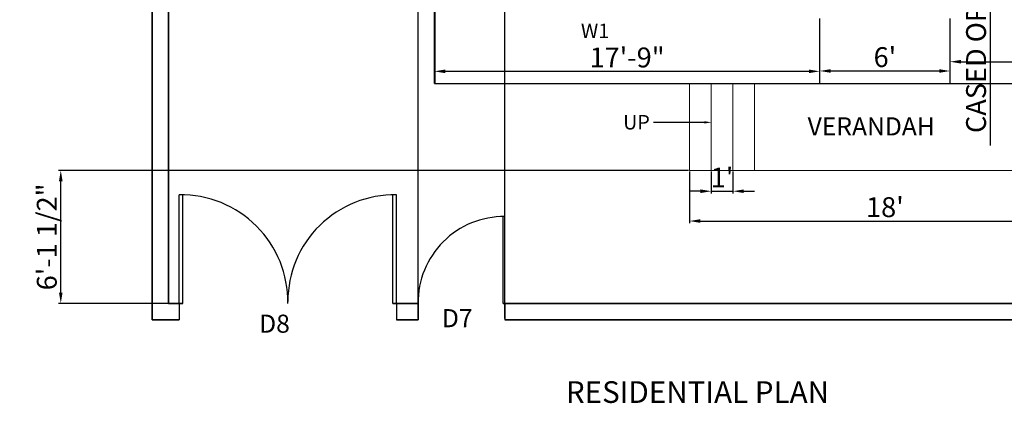
# Model space of a CAD drawing. Units: inches. Extents: x 2069 to 3028, y 691 to 1726.
# Tile 1 of 10: x 2069 to 2613, y 691 to 903. Entities that reach past the tile are written whole.
import ezdxf
from ezdxf import colors
from ezdxf.entities.mleader import LeaderData, LeaderLine
from ezdxf.math import Vec2, Vec3

# ---------------------------------------------------------------- set-up
doc = ezdxf.new("R2010")
doc.units = ezdxf.units.IN
for name, color, linetype, lineweight in [('A-ANNO-DIMS', 2, 'Continuous', 18), ('A-ANNO-TITL', 6, 'Continuous', 35), ('A-FLOR', 7, 'Continuous', 25), ('A-FLOR-STRS', 7, 'Continuous', 20), ('A-WALL', 7, 'Continuous', 40), ('L-SITE-GATE', 3, 'Continuous', 25), ('L-SITE-WALL', 7, 'Continuous', 35)]:
    doc.layers.add(name, color=color, linetype=linetype, lineweight=lineweight)
doc.layers.add('A-ANNO-TEXT', color=11, linetype='Continuous', lineweight=18, true_color=0xf27172)
doc.layers.add('A-AREA-IDEN', color=11, linetype='Continuous', lineweight=25, true_color=0xf27172)
doc.styles.get("Standard").update_dxf_attribs({"font": 'arial.ttf'})
doc.dimstyles.new('ISO-25', dxfattribs={"dimtxt": 11, "dimasz": 6, "dimexe": 1.25, "dimexo": 0.625, "dimtad": 1, "dimlunit": 3, "dimtxsty": 'Standard', "dimcen": 2.5, "dimclrd": 3, "dimclre": 5, "dimclrt": 6, "dimadec": 0, "dimazin": 0, "dimtfac": 1, "dimtmove": 0, "dimatfit": 3, "dimfxl": 1, "dimarcsym": 0})

# ---------------------------------------------------------------- blocks, each defined once
blk = doc.blocks.new('*D28')
at = {"layer": 'A-ANNO-DIMS', "color": 0, "lineweight": -2, "transparency": 16777216}
for p, q in [((2582.95, 868.51), (2582.95, 881.23)), ((2588.95, 879.98), (2789.95, 879.98)), ((2795.95, 868.51), (2795.95, 881.23))]:
    blk.add_line(p, q, dxfattribs=at)
at = {"layer": 'A-ANNO-DIMS', "color": 0, "transparency": 16777216}
for points in [[(2588.95, 880.98), (2588.95, 878.98), (2582.95, 879.98)], [(2789.95, 880.98), (2789.95, 878.98), (2795.95, 879.98)]]:
    blk.add_solid(points, dxfattribs=at)
at = {"layer": 'Defpoints', "color": 0, "transparency": 16777216}
for p in [(2795.95, 879.98), (2582.95, 867.89), (2795.95, 867.89)]:
    blk.add_point(p, dxfattribs=at)
at = {"layer": 'A-ANNO-DIMS', "color": 0, "transparency": 16777216, "insert": (2689.45, 886.22), "char_height": 11, "attachment_point": 5}
blk.add_mtext('17\'-9"', dxfattribs=at)
blk = doc.blocks.new('*D29')
at = {"layer": 'A-ANNO-DIMS', "color": 0, "lineweight": -2, "transparency": 16777216}
for p, q in [((2510.95, 868.51), (2510.95, 876.12)), ((2516.95, 874.87), (2576.95, 874.87)), ((2582.95, 868.51), (2582.95, 876.12))]:
    blk.add_line(p, q, dxfattribs=at)
at = {"layer": 'A-ANNO-DIMS', "color": 0, "transparency": 16777216}
for points in [[(2516.95, 875.87), (2516.95, 873.87), (2510.95, 874.87)], [(2576.95, 875.87), (2576.95, 873.87), (2582.95, 874.87)]]:
    blk.add_solid(points, dxfattribs=at)
at = {"layer": 'Defpoints', "color": 0, "transparency": 16777216}
for p in [(2582.95, 874.87), (2510.95, 867.89), (2582.95, 867.89)]:
    blk.add_point(p, dxfattribs=at)
at = {"layer": 'A-ANNO-DIMS', "color": 0, "transparency": 16777216, "insert": (2546.95, 881.11), "char_height": 11, "attachment_point": 5}
blk.add_mtext("6'", dxfattribs=at)
blk = doc.blocks.new('*D30')
at = {"layer": 'A-ANNO-DIMS', "color": 0, "lineweight": -2, "transparency": 16777216}
for p, q in [((2297.95, 868.51), (2297.95, 875.93)), ((2303.95, 874.68), (2504.95, 874.68)), ((2510.95, 868.51), (2510.95, 875.93))]:
    blk.add_line(p, q, dxfattribs=at)
at = {"layer": 'A-ANNO-DIMS', "color": 0, "transparency": 16777216}
for points in [[(2303.95, 875.68), (2303.95, 873.68), (2297.95, 874.68)], [(2504.95, 875.68), (2504.95, 873.68), (2510.95, 874.68)]]:
    blk.add_solid(points, dxfattribs=at)
at = {"layer": 'Defpoints', "color": 0, "transparency": 16777216}
for p in [(2510.95, 874.68), (2297.95, 867.89), (2510.95, 867.89)]:
    blk.add_point(p, dxfattribs=at)
at = {"layer": 'A-ANNO-DIMS', "color": 0, "transparency": 16777216, "insert": (2404.45, 880.92), "char_height": 11, "attachment_point": 5}
blk.add_mtext('17\'-9"', dxfattribs=at)
blk = doc.blocks.new('*D31')
at = {"layer": 'A-ANNO-DIMS', "color": 0, "lineweight": -2, "transparency": 16777216}
for p, q in [((2450.95, 819.26), (2450.95, 807.15)), ((2462.95, 819.26), (2462.95, 807.15)), ((2444.95, 808.4), (2438.95, 808.4)), ((2450.95, 808.4), (2462.95, 808.4)), ((2468.95, 808.4), (2474.95, 808.4))]:
    blk.add_line(p, q, dxfattribs=at)
at = {"layer": 'A-ANNO-DIMS', "color": 0, "transparency": 16777216}
for points in [[(2444.95, 809.4), (2444.95, 807.4), (2450.95, 808.4)], [(2468.95, 809.4), (2468.95, 807.4), (2462.95, 808.4)]]:
    blk.add_solid(points, dxfattribs=at)
at = {"layer": 'Defpoints', "color": 0, "transparency": 16777216}
for p in [(2450.95, 819.89), (2462.95, 819.89), (2462.95, 808.4)]:
    blk.add_point(p, dxfattribs=at)
at = {"layer": 'A-ANNO-DIMS', "color": 0, "transparency": 16777216, "insert": (2456.95, 814.55), "char_height": 11, "attachment_point": 5}
blk.add_mtext("1'", dxfattribs=at)
blk = doc.blocks.new('*D32')
at = {"layer": 'A-ANNO-DIMS', "color": 0, "lineweight": -2, "transparency": 16777216}
for p, q in [((2438.95, 819.26), (2438.95, 790.68)), ((2654.95, 819.26), (2654.95, 790.68)), ((2444.95, 791.93), (2648.95, 791.93))]:
    blk.add_line(p, q, dxfattribs=at)
at = {"layer": 'A-ANNO-DIMS', "color": 0, "transparency": 16777216}
for points in [[(2444.95, 792.93), (2444.95, 790.93), (2438.95, 791.93)], [(2648.95, 792.93), (2648.95, 790.93), (2654.95, 791.93)]]:
    blk.add_solid(points, dxfattribs=at)
at = {"layer": 'Defpoints', "color": 0, "transparency": 16777216}
for p in [(2438.95, 819.89), (2654.95, 819.89), (2654.95, 791.93)]:
    blk.add_point(p, dxfattribs=at)
at = {"layer": 'A-ANNO-DIMS', "color": 0, "transparency": 16777216, "insert": (2546.95, 798.17), "char_height": 11, "attachment_point": 5}
blk.add_mtext("18'", dxfattribs=at)
blk = doc.blocks.new('GATE-DOUBLE-120IN')
for p, q in [((0, 0), (0, 60)), ((2, 0), (2, 60)), ((118, 0), (118, 60)), ((120, 0), (120, 60)), ((0, 0), (0, -9)), ((120, 0), (120, -9))]:
    blk.add_line(p, q)
for centre, radius, start, end in [((1, 1), 59.01, 359.029, 90.971), ((119, 1.02), 58.99, 89.0287, 180.0165)]:
    blk.add_arc(centre, radius, start, end)
blk = doc.blocks.new('*D72')
at = {"layer": 'A-ANNO-DIMS', "color": 5, "lineweight": -2, "transparency": 16777216}
for p, q in [((2621.33, 1178.39), (2603.83, 1178.39)), ((2621.33, 1065.89), (2603.83, 1065.89))]:
    blk.add_line(p, q, dxfattribs=at)
at = {"layer": 'A-ANNO-DIMS', "color": 3, "lineweight": -2, "transparency": 16777216}
for p, q in [((2605.08, 1172.39), (2605.08, 1071.89)), ((2605.08, 1065.89), (2605.08, 833.73))]:
    blk.add_line(p, q, dxfattribs=at)
at = {"layer": 'A-ANNO-DIMS', "color": 3, "transparency": 16777216}
for points in [[(2604.08, 1172.39), (2606.08, 1172.39), (2605.08, 1178.39)], [(2604.08, 1071.89), (2606.08, 1071.89), (2605.08, 1065.89)]]:
    blk.add_solid(points, dxfattribs=at)
at = {"layer": 'Defpoints', "color": 0, "transparency": 16777216}
for p in [(2621.95, 1178.39), (2605.08, 1065.89), (2621.95, 1065.89)]:
    blk.add_point(p, dxfattribs=at)
at = {"layer": 'A-ANNO-DIMS', "color": 6, "transparency": 16777216, "insert": (2598.76, 946.81), "char_height": 11, "attachment_point": 5, "rotation": 90}
blk.add_mtext('CASED OPENING 9\'-4 1/2" TYP.', dxfattribs=at)
blk = doc.blocks.new('*D88')
at = {"layer": 'A-ANNO-DIMS', "color": 5, "lineweight": -2, "transparency": 16777216}
for p, q in [((2288.92, 738.01), (2288.92, 1704.14)), ((2336.92, 738.01), (2336.92, 1704.14))]:
    blk.add_line(p, q, dxfattribs=at)
at = {"layer": 'A-ANNO-DIMS', "color": 3, "lineweight": -2, "transparency": 16777216}
blk.add_line((2294.92, 1702.89), (2330.92, 1702.89), dxfattribs=at)
at = {"layer": 'A-ANNO-DIMS', "color": 3, "transparency": 16777216}
for points in [[(2294.92, 1703.89), (2294.92, 1701.89), (2288.92, 1702.89)], [(2330.92, 1703.89), (2330.92, 1701.89), (2336.92, 1702.89)]]:
    blk.add_solid(points, dxfattribs=at)
at = {"layer": 'Defpoints', "color": 0, "transparency": 16777216}
for p in [(2336.92, 1702.89), (2288.92, 737.39), (2336.92, 737.39)]:
    blk.add_point(p, dxfattribs=at)
at = {"layer": 'A-ANNO-DIMS', "color": 6, "transparency": 16777216, "insert": (2312.92, 1709.13), "char_height": 11, "attachment_point": 5}
blk.add_mtext('4\'-0"', dxfattribs=at)
blk = doc.blocks.new('*D89')
at = {"layer": 'A-ANNO-DIMS', "color": 5, "lineweight": -2, "transparency": 16777216}
for p, q in [((2336.92, 747.01), (2336.92, 1704.14)), ((2711.95, 747.01), (2711.95, 1704.14))]:
    blk.add_line(p, q, dxfattribs=at)
at = {"layer": 'A-ANNO-DIMS', "color": 3, "lineweight": -2, "transparency": 16777216}
blk.add_line((2342.92, 1702.89), (2705.95, 1702.89), dxfattribs=at)
at = {"layer": 'A-ANNO-DIMS', "color": 3, "transparency": 16777216}
for points in [[(2342.92, 1703.89), (2342.92, 1701.89), (2336.92, 1702.89)], [(2705.95, 1703.89), (2705.95, 1701.89), (2711.95, 1702.89)]]:
    blk.add_solid(points, dxfattribs=at)
at = {"layer": 'Defpoints', "color": 0, "transparency": 16777216}
for p in [(2711.95, 1702.89), (2336.92, 746.39), (2711.95, 746.39)]:
    blk.add_point(p, dxfattribs=at)
at = {"layer": 'A-ANNO-DIMS', "color": 6, "transparency": 16777216, "insert": (2524.44, 1709.13), "char_height": 11, "attachment_point": 5}
blk.add_mtext('31\'-3"', dxfattribs=at)
blk = doc.blocks.new('*D90')
at = {"layer": 'A-ANNO-DIMS', "color": 5, "lineweight": -2, "transparency": 16777216}
for p, q in [((2438.33, 819.89), (2090.2, 819.89)), ((2156.29, 746.39), (2090.2, 746.39))]:
    blk.add_line(p, q, dxfattribs=at)
at = {"layer": 'A-ANNO-DIMS', "color": 3, "lineweight": -2, "transparency": 16777216}
blk.add_line((2091.45, 752.39), (2091.45, 813.89), dxfattribs=at)
at = {"layer": 'A-ANNO-DIMS', "color": 3, "transparency": 16777216}
for points in [[(2090.45, 813.89), (2092.45, 813.89), (2091.45, 819.89)], [(2090.45, 752.39), (2092.45, 752.39), (2091.45, 746.39)]]:
    blk.add_solid(points, dxfattribs=at)
at = {"layer": 'Defpoints', "color": 0, "transparency": 16777216}
for p in [(2091.45, 819.89), (2438.95, 819.89), (2156.92, 746.39)]:
    blk.add_point(p, dxfattribs=at)
at = {"layer": 'A-ANNO-DIMS', "color": 6, "transparency": 16777216, "insert": (2085.14, 783.14), "char_height": 11, "attachment_point": 5, "rotation": 90}
blk.add_mtext('6\'-1 1/2"', dxfattribs=at)

msp = doc.modelspace()

# ---------------------------------------------------------------- linework, layer by layer
at = {"layer": 'A-FLOR'}
for p, q in [((2510.951, 867.887), (2510.951, 903.887)), ((2582.951, 867.887), (2582.951, 903.887)), ((2297.951, 867.887), (2795.951, 867.887)), ((2546.951, 867.887), (2582.951, 867.887))]:
    msp.add_line(p, q, dxfattribs=at)
at = {"layer": 'A-FLOR-STRS'}
for p, q in [((2438.951, 819.887), (2438.951, 867.887)), ((2450.951, 819.887), (2450.951, 867.887)), ((2462.951, 819.887), (2462.951, 867.887)), ((2474.951, 819.887), (2474.951, 867.887)), ((2438.951, 819.887), (2654.951, 819.887))]:
    msp.add_line(p, q, dxfattribs=at)
at = {"layer": 'A-WALL'}
msp.add_line((2297.951, 1056.887), (2297.951, 867.887), dxfattribs=at)
at = {"layer": 'L-SITE-GATE'}
for p, q in [((2335.919, 746.387), (2335.919, 794.387)), ((2336.919, 746.387), (2336.919, 794.387)), ((2288.919, 746.387), (2288.919, 737.387)), ((2336.919, 746.387), (2336.919, 737.387))]:
    msp.add_line(p, q, dxfattribs=at)
msp.add_arc((2336.419, 746.887), 47.503, 89.39691, 180.60309, dxfattribs=at)
at = {"layer": 'L-SITE-WALL'}
for p, q in [((2141.951, 1652.387), (2141.951, 737.387)), ((2150.951, 1535.387), (2150.951, 746.387)), ((2150.951, 746.387), (2158.919, 746.387)), ((2274.919, 746.387), (2288.919, 746.387)), ((2335.919, 746.387), (2713.951, 746.387)), ((2141.951, 737.387), (2156.919, 737.387)), ((2276.919, 737.387), (2288.919, 737.387)), ((2336.919, 737.387), (2711.951, 737.387))]:
    msp.add_line(p, q, dxfattribs=at)

# ---------------------------------------------------------------- block references
at = {"layer": 'L-SITE-GATE'}
msp.add_blockref('GATE-DOUBLE-120IN', (2156.919, 746.387), dxfattribs=at)

# ---------------------------------------------------------------- texts
at = {"layer": 'A-ANNO-TEXT', "attachment_point": 1}
for s, insert, char_height in [('{\\fArial|b1|i0|c0|p34;W1}', (2378.94, 901.037), 8), ('{\\fArial|b1|i0|c0|p34;D8}', (2201.103, 740.173), 10), ('{\\fArial|b1|i0|c0|p34;D7}', (2302.115, 743.208), 10)]:
    msp.add_mtext_dynamic_manual_height_columns(s, width=34.05605, gutter_width=12.5, heights=[0], dxfattribs=dict(at, insert=insert, char_height=char_height))
at = {"layer": 'A-ANNO-TITL', "insert": (2370.603, 703.362), "char_height": 12, "attachment_point": 1}
msp.add_mtext_dynamic_manual_height_columns('{\\fArial|b1|i0|c0|p34;RESIDENTIAL PLAN}', width=286.58107, gutter_width=12.5, heights=[0], dxfattribs=at)
at = {"layer": 'A-AREA-IDEN', "insert": (2504.232, 849.25), "char_height": 10, "attachment_point": 1}
msp.add_mtext_dynamic_manual_height_columns('VERANDAH', width=119.20948, gutter_width=12.5, heights=[21.969], dxfattribs=at)

# ---------------------------------------------------------------- dimensions: what is measured, and where the dimension line sits
at = {"layer": 'A-ANNO-DIMS'}
for base, p1, p2, override, picture, middle in [((2336.919, 1702.887), (2288.919, 737.387), (2336.919, 737.387), {"dimdec": 1, "dimlfac": 1, "dimrnd": 0, "dimzin": 1, "dimdsep": 46, "dimlunit": 4, "dimfrac": 2}, '*D88', (2312.919, 1709.128)), ((2711.951, 1702.887), (2336.919, 746.387), (2711.951, 746.387), {"dimdec": 1, "dimlfac": 1, "dimrnd": 0, "dimzin": 1, "dimdsep": 46, "dimlunit": 4, "dimfrac": 2}, '*D89', (2524.435, 1709.132)), ((2795.951, 879.977), (2582.951, 867.887), (2795.951, 867.887), {"dimclrd": 0, "dimclre": 0, "dimclrt": 0}, '*D28', (2689.451, 886.219)), ((2510.951, 874.681), (2297.951, 867.887), (2510.951, 867.887), {"dimclrd": 0, "dimclre": 0, "dimclrt": 0}, '*D30', (2404.451, 880.922)), ((2582.951, 874.869), (2510.951, 867.887), (2582.951, 867.887), {"dimclrd": 0, "dimclre": 0, "dimclrt": 0}, '*D29', (2546.951, 881.111)), ((2462.951, 808.404), (2450.951, 819.887), (2462.951, 819.887), {"dimclrd": 0, "dimclre": 0, "dimclrt": 0}, '*D31', (2456.951, 814.552)), ((2654.951, 791.93), (2438.951, 819.887), (2654.951, 819.887), {"dimclrd": 0, "dimclre": 0, "dimclrt": 0}, '*D32', (2546.951, 798.172))]:
    dim = msp.add_linear_dim(base=base, p1=p1, p2=p2, dimstyle='ISO-25', override=override, dxfattribs=at)
    dim.commit()
    dim.dimension.update_dxf_attribs({"geometry": picture, "text_midpoint": middle})
dim = msp.add_linear_dim(base=(2605.076, 1065.887), p1=(2621.951, 1178.387), p2=(2621.951, 1065.887), angle=270, text='CASED OPENING <> TYP.', dimstyle='ISO-25', override={"dimdec": 1, "dimlfac": 1, "dimrnd": 0, "dimzin": 1, "dimdsep": 46, "dimlunit": 4, "dimfrac": 2}, dxfattribs=at)
dim.commit()
dim.dimension.update_dxf_attribs({"geometry": '*D72', "text_midpoint": (2598.76, 946.808)})
dim = msp.add_linear_dim(base=(2091.451, 819.887), p1=(2156.919, 746.387), p2=(2438.951, 819.887), angle=90, dimstyle='ISO-25', override={"dimdec": 1, "dimlfac": 1, "dimrnd": 0, "dimzin": 1, "dimdsep": 46, "dimlunit": 4, "dimfrac": 2}, dxfattribs=at)
dim.commit()
dim.dimension.update_dxf_attribs({"geometry": '*D90', "text_midpoint": (2085.139, 783.137)})

# ---------------------------------------------------------------- leaders
at = {"layer": 'A-ANNO-TEXT'}
ml = msp.add_multileader_mtext('Standard', dxfattribs=at)
ml.set_content('UP', color=256)
ml.set_leader_properties()
ml.build(insert=Vec2(0, 0))
ctx = ml.context
ctx.base_point, ctx.char_height, ctx.plane_origin = Vec3(2400.858, 846.462), 8, Vec3(2451.166, 846.462)
ctx.text_align_type = 2
notes = []
notes.append((ctx, [(0, (1, 1, 0), (2427.019, 846.462), (-1, 0), 8, [(0, [(2451.166, 846.462)], 0, [])])]))
ctx.mtext.insert, ctx.mtext.width, ctx.mtext.alignment, ctx.mtext.flow_direction = Vec3(2417.019, 850.53), 13.45774, 3, 5
for ctx, leaders in notes:
    for number, flags, end, landing, length, lines in leaders:
        leader = LeaderData()
        leader.index, (leader.has_last_leader_line, leader.has_dogleg_vector, leader.attachment_direction) = number, flags
        leader.last_leader_point, leader.dogleg_vector, leader.dogleg_length = Vec3(end), Vec3(landing), length
        for number, points, colour, breaks in lines:
            line = LeaderLine()
            line.index, line.vertices, line.color, line.breaks = number, Vec3.list(points), colors.encode_raw_color(colour), breaks
            leader.lines.append(line)
        ctx.leaders.append(leader)

doc.saveas('drawing.dxf')
